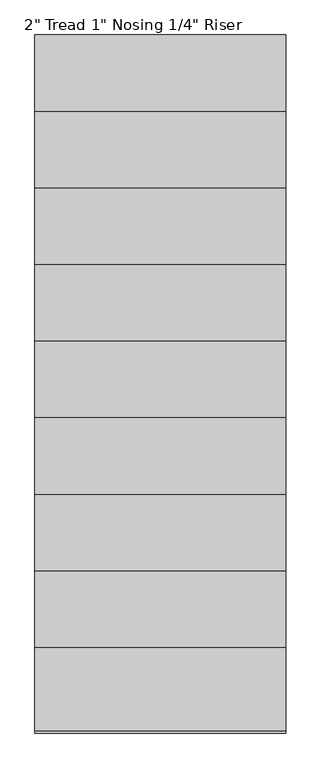
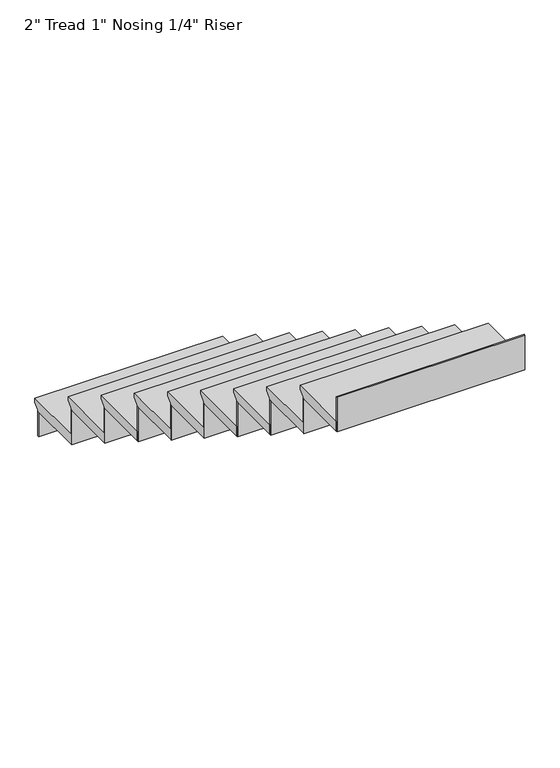
"""IFC4 building model written with IfcOpenShell, lengths in millimetres: stair flight geometry."""

from ifc_helpers import new_model, si_unit, origin, place, context, project, spatial, faceted_brep, source, transform, mapped, element, save


def stair_flight_731070e0(model_context):
    return source(origin(), model_context, "Body", "Brep", [
        faceted_brep([(14236.5506237, -1074.7064015, 3968.75), (14236.5506237, -1074.7064015, 3987.8), (15150.9506237, -1074.7064015, 3987.8), (15150.9506237, -1074.7064015, 3968.75), (14236.5506237, -1100.1064015, 3943.35), (15150.9506237, -1100.1064015, 3943.35), (14236.5506237, -1379.5064015, 3987.8), (15150.9506237, -1379.5064015, 3987.8), (15150.9506237, -1100.1064015, 3937.0), (15150.9506237, -1379.5064015, 3937.0), (14236.5506237, -1379.5064015, 3937.0), (14236.5506237, -1100.1064015, 3937.0)], [[[0, 1, 2, 3]], [[4, 0, 3, 5]], [[2, 1, 6, 7]], [[8, 9, 10, 11]], [[2, 7, 9, 8, 5, 3]], [[8, 11, 4, 5]], [[6, 1, 0, 4, 11, 10]], [[7, 6, 10, 9]]]),
        faceted_brep([(14236.5506237, -1100.1064015, 3937.0), (14236.5506237, -1100.1064015, 3810.0), (14236.5506237, -1106.4564015, 3810.0), (14236.5506237, -1106.4564015, 3937.0), (15150.9506237, -1100.1064015, 3937.0), (15150.9506237, -1106.4564015, 3937.0), (15150.9506237, -1106.4564015, 3810.0), (15150.9506237, -1100.1064015, 3810.0)], [[[0, 1, 2, 3]], [[4, 5, 6, 7]], [[1, 0, 4, 7]], [[2, 1, 7, 6]], [[3, 2, 6, 5]], [[0, 3, 5, 4]]]),
        faceted_brep([(14236.5506237, -1379.5064015, 4114.8), (14236.5506237, -1379.5064015, 3937.0), (14236.5506237, -1385.8564015, 3937.0), (14236.5506237, -1385.8564015, 4114.8), (15150.9506237, -1379.5064015, 4114.8), (15150.9506237, -1385.8564015, 4114.8), (15150.9506237, -1385.8564015, 3937.0), (15150.9506237, -1379.5064015, 3937.0)], [[[0, 1, 2, 3]], [[4, 5, 6, 7]], [[1, 0, 4, 7]], [[2, 1, 7, 6]], [[3, 2, 6, 5]], [[0, 3, 5, 4]]]),
        faceted_brep([(15150.9506237, -1354.1064015, 4165.6), (14236.5506237, -1354.1064015, 4165.6), (14236.5506237, -1658.9064015, 4165.6), (15150.9506237, -1658.9064015, 4165.6), (15150.9506237, -1379.5064015, 4114.8), (15150.9506237, -1658.9064015, 4114.8), (14236.5506237, -1658.9064015, 4114.8), (14236.5506237, -1379.5064015, 4114.8), (15150.9506237, -1379.5064015, 4121.15), (15150.9506237, -1354.1064015, 4146.55), (14236.5506237, -1379.5064015, 4121.15), (14236.5506237, -1354.1064015, 4146.55)], [[[0, 1, 2, 3]], [[4, 5, 6, 7]], [[0, 3, 5, 4, 8, 9]], [[4, 7, 10, 8]], [[2, 1, 11, 10, 7, 6]], [[3, 2, 6, 5]], [[11, 1, 0, 9]], [[10, 11, 9, 8]]]),
        faceted_brep([(14236.5506237, -1658.9064015, 4292.6), (14236.5506237, -1658.9064015, 4114.8), (14236.5506237, -1665.2564015, 4114.8), (14236.5506237, -1665.2564015, 4292.6), (15150.9506237, -1658.9064015, 4292.6), (15150.9506237, -1665.2564015, 4292.6), (15150.9506237, -1665.2564015, 4114.8), (15150.9506237, -1658.9064015, 4114.8)], [[[0, 1, 2, 3]], [[4, 5, 6, 7]], [[1, 0, 4, 7]], [[2, 1, 7, 6]], [[3, 2, 6, 5]], [[0, 3, 5, 4]]]),
        faceted_brep([(15150.9506237, -1633.5064015, 4343.4), (14236.5506237, -1633.5064015, 4343.4), (14236.5506237, -1938.3064015, 4343.4), (15150.9506237, -1938.3064015, 4343.4), (15150.9506237, -1658.9064015, 4292.6), (15150.9506237, -1938.3064015, 4292.6), (14236.5506237, -1938.3064015, 4292.6), (14236.5506237, -1658.9064015, 4292.6), (15150.9506237, -1658.9064015, 4298.95), (15150.9506237, -1633.5064015, 4324.35), (14236.5506237, -1658.9064015, 4298.95), (14236.5506237, -1633.5064015, 4324.35)], [[[0, 1, 2, 3]], [[4, 5, 6, 7]], [[0, 3, 5, 4, 8, 9]], [[4, 7, 10, 8]], [[2, 1, 11, 10, 7, 6]], [[3, 2, 6, 5]], [[11, 1, 0, 9]], [[10, 11, 9, 8]]]),
        faceted_brep([(14236.5506237, -1938.3064015, 4470.4), (14236.5506237, -1938.3064015, 4292.6), (14236.5506237, -1944.6564015, 4292.6), (14236.5506237, -1944.6564015, 4470.4), (15150.9506237, -1938.3064015, 4470.4), (15150.9506237, -1944.6564015, 4470.4), (15150.9506237, -1944.6564015, 4292.6), (15150.9506237, -1938.3064015, 4292.6)], [[[0, 1, 2, 3]], [[4, 5, 6, 7]], [[1, 0, 4, 7]], [[2, 1, 7, 6]], [[3, 2, 6, 5]], [[0, 3, 5, 4]]]),
        faceted_brep([(15150.9506237, -1912.9064015, 4521.2), (14236.5506237, -1912.9064015, 4521.2), (14236.5506237, -2217.7064015, 4521.2), (15150.9506237, -2217.7064015, 4521.2), (15150.9506237, -1938.3064015, 4470.4), (15150.9506237, -2217.7064015, 4470.4), (14236.5506237, -2217.7064015, 4470.4), (14236.5506237, -1938.3064015, 4470.4), (15150.9506237, -1938.3064015, 4476.75), (15150.9506237, -1912.9064015, 4502.15), (14236.5506237, -1938.3064015, 4476.75), (14236.5506237, -1912.9064015, 4502.15)], [[[0, 1, 2, 3]], [[4, 5, 6, 7]], [[0, 3, 5, 4, 8, 9]], [[4, 7, 10, 8]], [[2, 1, 11, 10, 7, 6]], [[3, 2, 6, 5]], [[11, 1, 0, 9]], [[10, 11, 9, 8]]]),
        faceted_brep([(14236.5506237, -2217.7064015, 4648.2), (14236.5506237, -2217.7064015, 4470.4), (14236.5506237, -2224.0564015, 4470.4), (14236.5506237, -2224.0564015, 4648.2), (15150.9506237, -2217.7064015, 4648.2), (15150.9506237, -2224.0564015, 4648.2), (15150.9506237, -2224.0564015, 4470.4), (15150.9506237, -2217.7064015, 4470.4)], [[[0, 1, 2, 3]], [[4, 5, 6, 7]], [[1, 0, 4, 7]], [[2, 1, 7, 6]], [[3, 2, 6, 5]], [[0, 3, 5, 4]]]),
        faceted_brep([(15150.9506237, -2192.3064015, 4699.0), (14236.5506237, -2192.3064015, 4699.0), (14236.5506237, -2497.1064015, 4699.0), (15150.9506237, -2497.1064015, 4699.0), (15150.9506237, -2217.7064015, 4648.2), (15150.9506237, -2497.1064015, 4648.2), (14236.5506237, -2497.1064015, 4648.2), (14236.5506237, -2217.7064015, 4648.2), (15150.9506237, -2217.7064015, 4654.55), (15150.9506237, -2192.3064015, 4679.95), (14236.5506237, -2217.7064015, 4654.55), (14236.5506237, -2192.3064015, 4679.95)], [[[0, 1, 2, 3]], [[4, 5, 6, 7]], [[0, 3, 5, 4, 8, 9]], [[4, 7, 10, 8]], [[2, 1, 11, 10, 7, 6]], [[3, 2, 6, 5]], [[11, 1, 0, 9]], [[10, 11, 9, 8]]]),
        faceted_brep([(14236.5506237, -2497.1064015, 4826.0), (14236.5506237, -2497.1064015, 4648.2), (14236.5506237, -2503.4564015, 4648.2), (14236.5506237, -2503.4564015, 4826.0), (15150.9506237, -2497.1064015, 4826.0), (15150.9506237, -2503.4564015, 4826.0), (15150.9506237, -2503.4564015, 4648.2), (15150.9506237, -2497.1064015, 4648.2)], [[[0, 1, 2, 3]], [[4, 5, 6, 7]], [[1, 0, 4, 7]], [[2, 1, 7, 6]], [[3, 2, 6, 5]], [[0, 3, 5, 4]]]),
        faceted_brep([(15150.9506237, -2471.7064015, 4876.8), (14236.5506237, -2471.7064015, 4876.8), (14236.5506237, -2776.5064015, 4876.8), (15150.9506237, -2776.5064015, 4876.8), (15150.9506237, -2497.1064015, 4826.0), (15150.9506237, -2776.5064015, 4826.0), (14236.5506237, -2776.5064015, 4826.0), (14236.5506237, -2497.1064015, 4826.0), (15150.9506237, -2497.1064015, 4832.35), (15150.9506237, -2471.7064015, 4857.75), (14236.5506237, -2497.1064015, 4832.35), (14236.5506237, -2471.7064015, 4857.75)], [[[0, 1, 2, 3]], [[4, 5, 6, 7]], [[0, 3, 5, 4, 8, 9]], [[4, 7, 10, 8]], [[2, 1, 11, 10, 7, 6]], [[3, 2, 6, 5]], [[11, 1, 0, 9]], [[10, 11, 9, 8]]]),
        faceted_brep([(14236.5506237, -2776.5064015, 5003.8), (14236.5506237, -2776.5064015, 4826.0), (14236.5506237, -2782.8564015, 4826.0), (14236.5506237, -2782.8564015, 5003.8), (15150.9506237, -2776.5064015, 5003.8), (15150.9506237, -2782.8564015, 5003.8), (15150.9506237, -2782.8564015, 4826.0), (15150.9506237, -2776.5064015, 4826.0)], [[[0, 1, 2, 3]], [[4, 5, 6, 7]], [[1, 0, 4, 7]], [[2, 1, 7, 6]], [[3, 2, 6, 5]], [[0, 3, 5, 4]]]),
        faceted_brep([(15150.9506237, -2751.1064015, 5054.6), (14236.5506237, -2751.1064015, 5054.6), (14236.5506237, -3055.9064015, 5054.6), (15150.9506237, -3055.9064015, 5054.6), (15150.9506237, -2776.5064015, 5003.8), (15150.9506237, -3055.9064015, 5003.8), (14236.5506237, -3055.9064015, 5003.8), (14236.5506237, -2776.5064015, 5003.8), (15150.9506237, -2776.5064015, 5010.15), (15150.9506237, -2751.1064015, 5035.55), (14236.5506237, -2776.5064015, 5010.15), (14236.5506237, -2751.1064015, 5035.55)], [[[0, 1, 2, 3]], [[4, 5, 6, 7]], [[0, 3, 5, 4, 8, 9]], [[4, 7, 10, 8]], [[2, 1, 11, 10, 7, 6]], [[3, 2, 6, 5]], [[11, 1, 0, 9]], [[10, 11, 9, 8]]]),
        faceted_brep([(14236.5506237, -3055.9064015, 5181.6), (14236.5506237, -3055.9064015, 5003.8), (14236.5506237, -3062.2564015, 5003.8), (14236.5506237, -3062.2564015, 5181.6), (15150.9506237, -3055.9064015, 5181.6), (15150.9506237, -3062.2564015, 5181.6), (15150.9506237, -3062.2564015, 5003.8), (15150.9506237, -3055.9064015, 5003.8)], [[[0, 1, 2, 3]], [[4, 5, 6, 7]], [[1, 0, 4, 7]], [[2, 1, 7, 6]], [[3, 2, 6, 5]], [[0, 3, 5, 4]]]),
        faceted_brep([(15150.9506237, -3030.5064015, 5232.4), (14236.5506237, -3030.5064015, 5232.4), (14236.5506237, -3335.3064015, 5232.4), (15150.9506237, -3335.3064015, 5232.4), (15150.9506237, -3055.9064015, 5181.6), (15150.9506237, -3335.3064015, 5181.6), (14236.5506237, -3335.3064015, 5181.6), (14236.5506237, -3055.9064015, 5181.6), (15150.9506237, -3055.9064015, 5187.95), (15150.9506237, -3030.5064015, 5213.35), (14236.5506237, -3055.9064015, 5187.95), (14236.5506237, -3030.5064015, 5213.35)], [[[0, 1, 2, 3]], [[4, 5, 6, 7]], [[0, 3, 5, 4, 8, 9]], [[4, 7, 10, 8]], [[2, 1, 11, 10, 7, 6]], [[3, 2, 6, 5]], [[11, 1, 0, 9]], [[10, 11, 9, 8]]]),
        faceted_brep([(14236.5506237, -3614.7064015, 5537.2), (14236.5506237, -3614.7064015, 5359.4), (14236.5506237, -3621.0564015, 5359.4), (14236.5506237, -3621.0564015, 5537.2), (15150.9506237, -3614.7064015, 5537.2), (15150.9506237, -3621.0564015, 5537.2), (15150.9506237, -3621.0564015, 5359.4), (15150.9506237, -3614.7064015, 5359.4)], [[[0, 1, 2, 3]], [[4, 5, 6, 7]], [[1, 0, 4, 7]], [[2, 1, 7, 6]], [[3, 2, 6, 5]], [[0, 3, 5, 4]]]),
        faceted_brep([(14236.5506237, -3335.3064015, 5359.4), (14236.5506237, -3335.3064015, 5181.6), (14236.5506237, -3341.6564015, 5181.6), (14236.5506237, -3341.6564015, 5359.4), (15150.9506237, -3335.3064015, 5359.4), (15150.9506237, -3341.6564015, 5359.4), (15150.9506237, -3341.6564015, 5181.6), (15150.9506237, -3335.3064015, 5181.6)], [[[0, 1, 2, 3]], [[4, 5, 6, 7]], [[1, 0, 4, 7]], [[2, 1, 7, 6]], [[3, 2, 6, 5]], [[0, 3, 5, 4]]]),
        faceted_brep([(15150.9506237, -3614.7064015, 5410.2), (15150.9506237, -3589.3064015, 5410.2), (15150.9506237, -3309.9064015, 5410.2), (14236.5506237, -3309.9064015, 5410.2), (14236.5506237, -3614.7064015, 5410.2), (15150.9506237, -3589.3064015, 5359.4), (15150.9506237, -3614.7064015, 5359.4), (14236.5506237, -3614.7064015, 5359.4), (14236.5506237, -3335.3064015, 5359.4), (15150.9506237, -3335.3064015, 5359.4), (15150.9506237, -3335.3064015, 5365.75), (15150.9506237, -3309.9064015, 5391.15), (14236.5506237, -3335.3064015, 5365.75), (14236.5506237, -3309.9064015, 5391.15)], [[[0, 1, 2, 3, 4]], [[5, 6, 7, 8, 9]], [[1, 0, 6, 5]], [[2, 1, 5, 9, 10, 11]], [[9, 8, 12, 10]], [[4, 3, 13, 12, 8, 7]], [[0, 4, 7, 6]], [[13, 3, 2, 11]], [[12, 13, 11, 10]]]),
    ])


if __name__ == "__main__":
    model = new_model("IFC4")
    model_context = context("Model", 3, world=origin())
    ifc_project = project(units=[si_unit("LENGTHUNIT", "METRE", prefix="MILLI")], contexts=[model_context])
    site = spatial("IfcSite", under=ifc_project)
    building = spatial("IfcBuilding", under=site)
    placement = place(None, origin())
    stair_flight_shape = stair_flight_731070e0(model_context)
    element("IfcStairFlight", 1, ObjectType="2\" Tread 1\" Nosing 1/4\" Riser", at=placement, inside=building, context=model_context, shape_type="MappedRepresentation", body=[
        mapped(stair_flight_shape, transform((0.0, 0.0, 0.0), x_axis=(1.0, 0.0, 0.0), y_axis=(0.0, 1.0, 0.0), z_axis=(0.0, 0.0, 1.0))),
    ])
    save(model, "model.ifc")
